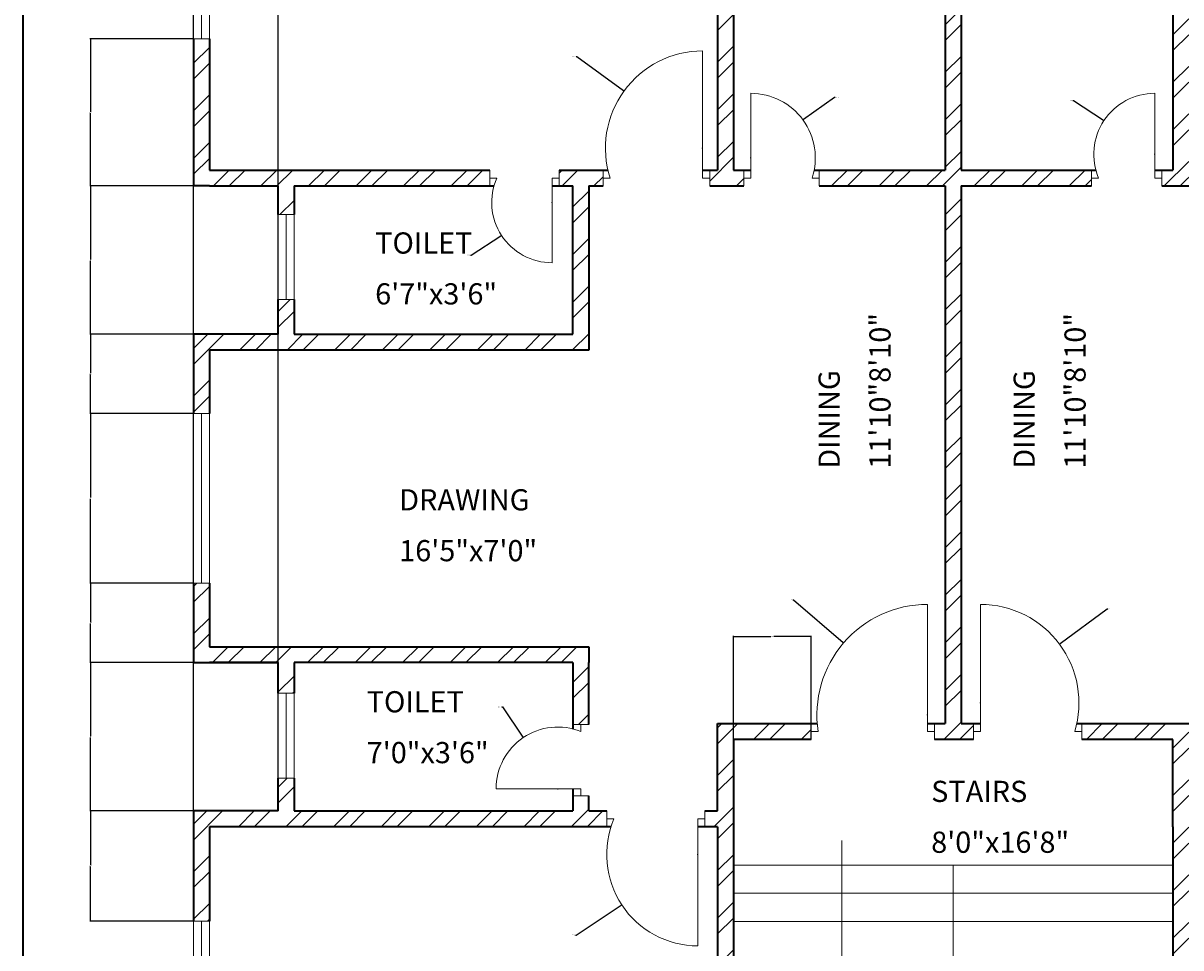
# Model space of a CAD drawing. Units: inches. Extents: x 2271 to 2815, y 1169 to 1838.
# Tile 2 of 4: x 2271 to 2599, y 1395 to 1657. Entities that reach past the tile are written whole.
import ezdxf

# ---------------------------------------------------------------- set-up
doc = ezdxf.new("R2010")
doc.units = ezdxf.units.IN
for name, color, linetype, lineweight in [('A-ANNO-DIMS', 2, 'Continuous', 18), ('A-ANNO-SYMB', 101, 'Continuous', 13), ('A-ANNO-TTLB', 7, 'Continuous', 35), ('A-AREA-IDEN', 7, 'Continuous', 18), ('A-DOOR', 11, 'Continuous', 18), ('A-FLOR-STRS', 101, 'Continuous', 18), ('A-GLAZ', 181, 'Continuous', 18), ('A-WALL', 7, 'Continuous', 35)]:
    doc.layers.add(name, color=color, linetype=linetype, lineweight=lineweight)
doc.layers.add('A-WALL-PATT', color=9, linetype='Continuous', lineweight=13, true_color=0xafd9aa)
doc.styles.get("Standard").update_dxf_attribs({"font": 'arial.ttf'})
doc.dimstyles.get("Standard").update_dxf_attribs({"dimtxt": 0.18, "dimasz": 0.18, "dimexe": 0.18, "dimexo": 0.0625, "dimgap": 0.09, "dimtad": 0, "dimtih": 1, "dimtoh": 1, "dimdec": 4, "dimzin": 0, "dimdsep": 46, "dimtxsty": 'Standard', "dimcen": 0.09, "dimadec": 0, "dimazin": 0, "dimtfac": 1, "dimtdec": 4, "dimtofl": 0, "dimtmove": 0, "dimatfit": 3, "dimfxl": 1, "dimtolj": 1, "dimtzin": 0, "dimarcsym": 0})

# ---------------------------------------------------------------- blocks, each defined once
blk = doc.blocks.new('WIN-60IN')
for p, q in [((0, 4.5), (0, 0)), ((60, 4.5), (0, 4.5)), ((60, 2.25), (60, 4.5)), ((60, 4.5), (60, 0)), ((0, 0), (0, 2.25)), ((0, 2.25), (60, 2.25)), ((0, 0), (60, 0))]:
    blk.add_line(p, q)
blk = doc.blocks.new('WIN-24IN')
for p, q in [((0, 4.5), (0, 0)), ((0, 4.5), (24, 4.5)), ((24, 2.25), (24, 4.5)), ((24, 4.5), (24, 0)), ((0, 0), (0, 2.25)), ((0, 2.25), (24, 2.25)), ((24, 0), (0, 0))]:
    blk.add_line(p, q)
blk = doc.blocks.new('*D14')
at = {"layer": 'A-ANNO-DIMS', "color": 0, "lineweight": -2, "transparency": 16777216}
for p, q in [((2318.74, 1433.53), (2289.47, 1433.53)), ((2289.65, 1433.35), (2289.65, 1418.1)), ((2289.65, 1402.49), (2289.65, 1417.74)), ((2318.74, 1402.31), (2289.47, 1402.31))]:
    blk.add_line(p, q, dxfattribs=at)
at = {"layer": 'A-ANNO-DIMS', "color": 0, "transparency": 16777216}
for points in [[(2289.62, 1433.35), (2289.68, 1433.35), (2289.65, 1433.53)], [(2289.62, 1402.49), (2289.68, 1402.49), (2289.65, 1402.31)]]:
    blk.add_solid(points, dxfattribs=at)
at = {"layer": 'Defpoints', "color": 0, "transparency": 16777216}
for p in [(2289.65, 1433.53), (2318.8, 1433.53), (2318.8, 1402.31)]:
    blk.add_point(p, dxfattribs=at)
at = {"layer": 'A-ANNO-DIMS', "color": 0, "transparency": 16777216, "insert": (2289.65, 1417.92), "char_height": 0.18, "attachment_point": 5}
blk.add_mtext('\\A1;31.22', dxfattribs=at)
blk = doc.blocks.new('*D15')
at = {"layer": 'A-ANNO-DIMS', "color": 0, "lineweight": -2, "transparency": 16777216}
for p, q in [((2318.74, 1475.53), (2289.47, 1475.53)), ((2289.65, 1475.35), (2289.65, 1454.71)), ((2289.65, 1433.71), (2289.65, 1454.35)), ((2318.74, 1433.53), (2289.47, 1433.53))]:
    blk.add_line(p, q, dxfattribs=at)
at = {"layer": 'A-ANNO-DIMS', "color": 0, "transparency": 16777216}
for points in [[(2289.62, 1475.35), (2289.68, 1475.35), (2289.65, 1475.53)], [(2289.62, 1433.71), (2289.68, 1433.71), (2289.65, 1433.53)]]:
    blk.add_solid(points, dxfattribs=at)
at = {"layer": 'Defpoints', "color": 0, "transparency": 16777216}
for p in [(2289.65, 1475.53), (2318.8, 1475.53), (2318.8, 1433.53)]:
    blk.add_point(p, dxfattribs=at)
at = {"layer": 'A-ANNO-DIMS', "color": 0, "transparency": 16777216, "insert": (2289.65, 1454.53), "char_height": 0.18, "attachment_point": 5}
blk.add_mtext('\\A1;42', dxfattribs=at)
blk = doc.blocks.new('*D16')
at = {"layer": 'A-ANNO-DIMS', "color": 0, "lineweight": -2, "transparency": 16777216}
for p, q in [((2318.74, 1498.07), (2289.47, 1498.07)), ((2289.65, 1497.89), (2289.65, 1486.98)), ((2289.65, 1475.71), (2289.65, 1486.62)), ((2318.74, 1475.53), (2289.47, 1475.53))]:
    blk.add_line(p, q, dxfattribs=at)
at = {"layer": 'A-ANNO-DIMS', "color": 0, "transparency": 16777216}
for points in [[(2289.62, 1497.89), (2289.68, 1497.89), (2289.65, 1498.07)], [(2289.62, 1475.71), (2289.68, 1475.71), (2289.65, 1475.53)]]:
    blk.add_solid(points, dxfattribs=at)
at = {"layer": 'Defpoints', "color": 0, "transparency": 16777216}
for p in [(2289.65, 1498.07), (2318.8, 1498.07), (2318.8, 1475.53)]:
    blk.add_point(p, dxfattribs=at)
at = {"layer": 'A-ANNO-DIMS', "color": 0, "transparency": 16777216, "insert": (2289.65, 1486.8), "char_height": 0.18, "attachment_point": 5}
blk.add_mtext('\\A1;22.54', dxfattribs=at)
blk = doc.blocks.new('*D17')
at = {"layer": 'A-ANNO-DIMS', "color": 0, "lineweight": -2, "transparency": 16777216}
for p, q in [((2318.74, 1546.07), (2289.47, 1546.07)), ((2289.65, 1545.89), (2289.65, 1522.25)), ((2289.65, 1498.25), (2289.65, 1521.89)), ((2318.74, 1498.07), (2289.47, 1498.07))]:
    blk.add_line(p, q, dxfattribs=at)
at = {"layer": 'A-ANNO-DIMS', "color": 0, "transparency": 16777216}
for points in [[(2289.62, 1545.89), (2289.68, 1545.89), (2289.65, 1546.07)], [(2289.62, 1498.25), (2289.68, 1498.25), (2289.65, 1498.07)]]:
    blk.add_solid(points, dxfattribs=at)
at = {"layer": 'Defpoints', "color": 0, "transparency": 16777216}
for p in [(2289.65, 1546.07), (2318.8, 1546.07), (2318.8, 1498.07)]:
    blk.add_point(p, dxfattribs=at)
at = {"layer": 'A-ANNO-DIMS', "color": 0, "transparency": 16777216, "insert": (2289.65, 1522.07), "char_height": 0.18, "attachment_point": 5}
blk.add_mtext('\\A1;48', dxfattribs=at)
blk = doc.blocks.new('*D18')
at = {"layer": 'A-ANNO-DIMS', "color": 0, "lineweight": -2, "transparency": 16777216}
for p, q in [((2318.74, 1568.53), (2289.47, 1568.53)), ((2289.65, 1568.35), (2289.65, 1557.48)), ((2289.65, 1546.25), (2289.65, 1557.12)), ((2318.74, 1546.07), (2289.47, 1546.07))]:
    blk.add_line(p, q, dxfattribs=at)
at = {"layer": 'A-ANNO-DIMS', "color": 0, "transparency": 16777216}
for points in [[(2289.62, 1568.35), (2289.68, 1568.35), (2289.65, 1568.53)], [(2289.62, 1546.25), (2289.68, 1546.25), (2289.65, 1546.07)]]:
    blk.add_solid(points, dxfattribs=at)
at = {"layer": 'Defpoints', "color": 0, "transparency": 16777216}
for p in [(2289.65, 1568.53), (2318.8, 1568.53), (2318.8, 1546.07)]:
    blk.add_point(p, dxfattribs=at)
at = {"layer": 'A-ANNO-DIMS', "color": 0, "transparency": 16777216, "insert": (2289.65, 1557.3), "char_height": 0.18, "attachment_point": 5}
blk.add_mtext('\\A1;22.46', dxfattribs=at)
blk = doc.blocks.new('*D19')
at = {"layer": 'A-ANNO-DIMS', "color": 0, "lineweight": -2, "transparency": 16777216}
for p, q in [((2318.74, 1610.53), (2289.47, 1610.53)), ((2289.65, 1610.35), (2289.65, 1589.71)), ((2289.65, 1568.71), (2289.65, 1589.35)), ((2318.74, 1568.53), (2289.47, 1568.53))]:
    blk.add_line(p, q, dxfattribs=at)
at = {"layer": 'A-ANNO-DIMS', "color": 0, "transparency": 16777216}
for points in [[(2289.62, 1610.35), (2289.68, 1610.35), (2289.65, 1610.53)], [(2289.62, 1568.71), (2289.68, 1568.71), (2289.65, 1568.53)]]:
    blk.add_solid(points, dxfattribs=at)
at = {"layer": 'Defpoints', "color": 0, "transparency": 16777216}
for p in [(2289.65, 1610.53), (2318.8, 1610.53), (2318.8, 1568.53)]:
    blk.add_point(p, dxfattribs=at)
at = {"layer": 'A-ANNO-DIMS', "color": 0, "transparency": 16777216, "insert": (2289.65, 1589.53), "char_height": 0.18, "attachment_point": 5}
blk.add_mtext('\\A1;42', dxfattribs=at)
blk = doc.blocks.new('*D20')
at = {"layer": 'A-ANNO-DIMS', "color": 0, "lineweight": -2, "transparency": 16777216}
for p, q in [((2318.74, 1652.22), (2289.47, 1652.22)), ((2289.65, 1652.04), (2289.65, 1631.56)), ((2289.65, 1610.71), (2289.65, 1631.19)), ((2318.74, 1610.53), (2289.47, 1610.53))]:
    blk.add_line(p, q, dxfattribs=at)
at = {"layer": 'A-ANNO-DIMS', "color": 0, "transparency": 16777216}
for points in [[(2289.62, 1652.04), (2289.68, 1652.04), (2289.65, 1652.22)], [(2289.62, 1610.71), (2289.68, 1610.71), (2289.65, 1610.53)]]:
    blk.add_solid(points, dxfattribs=at)
at = {"layer": 'Defpoints', "color": 0, "transparency": 16777216}
for p in [(2289.65, 1652.22), (2318.8, 1652.22), (2318.8, 1610.53)]:
    blk.add_point(p, dxfattribs=at)
at = {"layer": 'A-ANNO-DIMS', "color": 0, "transparency": 16777216, "insert": (2289.65, 1631.37), "char_height": 0.18, "attachment_point": 5}
blk.add_mtext('\\A1;41.69', dxfattribs=at)
blk = doc.blocks.new('*D23')
at = {"layer": 'A-ANNO-DIMS', "color": 0, "lineweight": -2, "transparency": 16777216}
for p, q in [((2318.8, 1433.59), (2318.8, 1816.86)), ((2318.98, 1816.68), (2330.58, 1816.68)), ((2342.62, 1816.68), (2331.02, 1816.68)), ((2342.8, 1433.59), (2342.8, 1816.86))]:
    blk.add_line(p, q, dxfattribs=at)
at = {"layer": 'A-ANNO-DIMS', "color": 0, "transparency": 16777216}
for points in [[(2318.98, 1816.71), (2318.98, 1816.65), (2318.8, 1816.68)], [(2342.62, 1816.71), (2342.62, 1816.65), (2342.8, 1816.68)]]:
    blk.add_solid(points, dxfattribs=at)
at = {"layer": 'Defpoints', "color": 0, "transparency": 16777216}
for p in [(2342.8, 1816.68), (2318.8, 1433.53), (2342.8, 1433.53)]:
    blk.add_point(p, dxfattribs=at)
at = {"layer": 'A-ANNO-DIMS', "color": 0, "transparency": 16777216, "insert": (2330.8, 1816.68), "char_height": 0.18, "attachment_point": 5}
blk.add_mtext('\\A1;24', dxfattribs=at)
blk = doc.blocks.new('*D36')
at = {"layer": 'A-ANNO-DIMS', "color": 0, "lineweight": -2, "transparency": 16777216}
for p, q in [((2471.8, 1453.82), (2471.8, 1483.08)), ((2471.98, 1482.9), (2482.4, 1482.9)), ((2493.61, 1482.9), (2483.19, 1482.9)), ((2493.79, 1453.82), (2493.79, 1483.08))]:
    blk.add_line(p, q, dxfattribs=at)
at = {"layer": 'A-ANNO-DIMS', "color": 0, "transparency": 16777216}
for points in [[(2471.98, 1482.93), (2471.98, 1482.87), (2471.8, 1482.9)], [(2493.61, 1482.93), (2493.61, 1482.87), (2493.79, 1482.9)]]:
    blk.add_solid(points, dxfattribs=at)
at = {"layer": 'Defpoints', "color": 0, "transparency": 16777216}
for p in [(2493.79, 1482.9), (2471.8, 1453.75), (2493.79, 1453.75)]:
    blk.add_point(p, dxfattribs=at)
at = {"layer": 'A-ANNO-DIMS', "color": 0, "transparency": 16777216, "insert": (2482.8, 1482.9), "char_height": 0.18, "attachment_point": 5}
blk.add_mtext('\\A1;21.99', dxfattribs=at)
blk = doc.blocks.new('*D37')
at = {"layer": 'A-ANNO-DIMS', "color": 0, "lineweight": -2, "transparency": 16777216}
for p, q in [((2488.58, 1493.35), (2488.76, 1493.35)), ((2488.76, 1493.35), (2502.87, 1481.23)), ((2526.65, 1460.7), (2526.83, 1460.7)), ((2526.74, 1460.61), (2526.74, 1460.79))]:
    blk.add_line(p, q, dxfattribs=at)
at = {"layer": 'A-ANNO-DIMS', "color": 0, "transparency": 16777216}
blk.add_solid([(2502.89, 1481.25), (2502.85, 1481.2), (2503, 1481.11)], dxfattribs=at)
at = {"layer": 'Defpoints', "color": 0, "transparency": 16777216}
for p in [(2503, 1481.11), (2526.74, 1460.7)]:
    blk.add_point(p, dxfattribs=at)
at = {"layer": 'A-ANNO-DIMS', "color": 0, "transparency": 16777216, "insert": (2488.03, 1493.35), "char_height": 0.18, "attachment_point": 5}
blk.add_mtext('\\A1;R31.305', dxfattribs=at)
blk = doc.blocks.new('*D38')
at = {"layer": 'A-ANNO-DIMS', "color": 0, "lineweight": -2, "transparency": 16777216}
for p, q in [((2577.64, 1490.7), (2564.34, 1480.83)), ((2577.82, 1490.7), (2577.64, 1490.7)), ((2541.69, 1464.1), (2541.87, 1464.1)), ((2541.78, 1464.01), (2541.78, 1464.19))]:
    blk.add_line(p, q, dxfattribs=at)
at = {"layer": 'A-ANNO-DIMS', "color": 0, "transparency": 16777216}
blk.add_solid([(2564.32, 1480.86), (2564.35, 1480.81), (2564.19, 1480.73)], dxfattribs=at)
at = {"layer": 'Defpoints', "color": 0, "transparency": 16777216}
for p in [(2564.19, 1480.73), (2541.78, 1464.1)]:
    blk.add_point(p, dxfattribs=at)
at = {"layer": 'A-ANNO-DIMS', "color": 0, "transparency": 16777216, "insert": (2578.23, 1490.7), "char_height": 0.18, "attachment_point": 5}
blk.add_mtext('\\A1;R27.9', dxfattribs=at)
blk = doc.blocks.new('*D39')
at = {"layer": 'A-ANNO-DIMS', "color": 0, "lineweight": -2, "transparency": 16777216}
for p, q in [((2427.25, 1647.18), (2427.43, 1647.18)), ((2427.43, 1647.18), (2440.65, 1637.56)), ((2462.97, 1621.24), (2463.15, 1621.24)), ((2463.06, 1621.15), (2463.06, 1621.33))]:
    blk.add_line(p, q, dxfattribs=at)
at = {"layer": 'A-ANNO-DIMS', "color": 0, "transparency": 16777216}
blk.add_solid([(2440.67, 1637.58), (2440.63, 1637.53), (2440.79, 1637.45)], dxfattribs=at)
at = {"layer": 'Defpoints', "color": 0, "transparency": 16777216}
for p in [(2440.79, 1637.45), (2463.06, 1621.24)]:
    blk.add_point(p, dxfattribs=at)
at = {"layer": 'A-ANNO-DIMS', "color": 0, "transparency": 16777216, "insert": (2426.7, 1647.18), "char_height": 0.18, "attachment_point": 5}
blk.add_mtext('\\A1;R27.546', dxfattribs=at)
blk = doc.blocks.new('*D41')
at = {"layer": 'A-ANNO-DIMS', "color": 0, "lineweight": -2, "transparency": 16777216}
for p, q in [((2461.62, 1421.13), (2461.8, 1421.13)), ((2461.71, 1421.04), (2461.71, 1421.22)), ((2427.2, 1398.34), (2439.99, 1406.79)), ((2427.02, 1398.34), (2427.2, 1398.34))]:
    blk.add_line(p, q, dxfattribs=at)
at = {"layer": 'A-ANNO-DIMS', "color": 0, "transparency": 16777216}
blk.add_solid([(2439.98, 1406.81), (2440.01, 1406.76), (2440.14, 1406.89)], dxfattribs=at)
at = {"layer": 'Defpoints', "color": 0, "transparency": 16777216}
for p in [(2461.71, 1421.13), (2440.14, 1406.89)]:
    blk.add_point(p, dxfattribs=at)
at = {"layer": 'A-ANNO-DIMS', "color": 0, "transparency": 16777216, "insert": (2426.47, 1398.34), "char_height": 0.18, "attachment_point": 5}
blk.add_mtext('\\A1;R25.845', dxfattribs=at)
blk = doc.blocks.new('*D47')
at = {"layer": 'A-ANNO-DIMS', "color": 0, "lineweight": -2, "transparency": 16777216}
for p, q in [((2500.41, 1635.64), (2491.67, 1629.32)), ((2500.59, 1635.64), (2500.41, 1635.64)), ((2476.63, 1618.51), (2476.81, 1618.51)), ((2476.72, 1618.42), (2476.72, 1618.6))]:
    blk.add_line(p, q, dxfattribs=at)
at = {"layer": 'A-ANNO-DIMS', "color": 0, "transparency": 16777216}
blk.add_solid([(2491.66, 1629.34), (2491.69, 1629.3), (2491.53, 1629.22)], dxfattribs=at)
at = {"layer": 'Defpoints', "color": 0, "transparency": 16777216}
for p in [(2491.53, 1629.22), (2476.72, 1618.51)]:
    blk.add_point(p, dxfattribs=at)
at = {"layer": 'A-ANNO-DIMS', "color": 0, "transparency": 16777216, "insert": (2501.14, 1635.64), "char_height": 0.18, "attachment_point": 5}
blk.add_mtext('\\A1;R18.274', dxfattribs=at)
blk = doc.blocks.new('*D49')
at = {"layer": 'A-ANNO-DIMS', "color": 0, "lineweight": -2, "transparency": 16777216}
for p, q in [((2406.19, 1462.97), (2406.37, 1462.97)), ((2406.37, 1462.97), (2412.14, 1454.42)), ((2421.95, 1439.79), (2422.13, 1439.79)), ((2422.04, 1439.7), (2422.04, 1439.88))]:
    blk.add_line(p, q, dxfattribs=at)
at = {"layer": 'A-ANNO-DIMS', "color": 0, "transparency": 16777216}
blk.add_solid([(2412.17, 1454.44), (2412.12, 1454.41), (2412.24, 1454.27)], dxfattribs=at)
at = {"layer": 'Defpoints', "color": 0, "transparency": 16777216}
for p in [(2412.24, 1454.27), (2422.04, 1439.79)]:
    blk.add_point(p, dxfattribs=at)
at = {"layer": 'A-ANNO-DIMS', "color": 0, "transparency": 16777216, "insert": (2405.64, 1462.97), "char_height": 0.18, "attachment_point": 5}
blk.add_mtext('\\A1;R17.485', dxfattribs=at)
blk = doc.blocks.new('*D51')
at = {"layer": 'A-ANNO-DIMS', "color": 0, "lineweight": -2, "transparency": 16777216}
for p, q in [((2567.95, 1634.76), (2568.13, 1634.76)), ((2568.13, 1634.76), (2576.61, 1629.15)), ((2591.06, 1619.53), (2591.24, 1619.53)), ((2591.15, 1619.44), (2591.15, 1619.62))]:
    blk.add_line(p, q, dxfattribs=at)
at = {"layer": 'A-ANNO-DIMS', "color": 0, "transparency": 16777216}
blk.add_solid([(2576.63, 1629.18), (2576.6, 1629.13), (2576.76, 1629.05)], dxfattribs=at)
at = {"layer": 'Defpoints', "color": 0, "transparency": 16777216}
for p in [(2576.76, 1629.05), (2591.15, 1619.53)]:
    blk.add_point(p, dxfattribs=at)
at = {"layer": 'A-ANNO-DIMS', "color": 0, "transparency": 16777216, "insert": (2567.47, 1634.76), "char_height": 0.18, "attachment_point": 5}
blk.add_mtext('\\A1;R17.25', dxfattribs=at)
blk = doc.blocks.new('*D52')
at = {"layer": 'A-ANNO-DIMS', "color": 0, "lineweight": -2, "transparency": 16777216}
for p, q in [((2420.3, 1605.88), (2420.48, 1605.88)), ((2420.39, 1605.79), (2420.39, 1605.97)), ((2397.48, 1590.94), (2405.92, 1596.45)), ((2397.3, 1590.94), (2397.48, 1590.94))]:
    blk.add_line(p, q, dxfattribs=at)
at = {"layer": 'A-ANNO-DIMS', "color": 0, "transparency": 16777216}
blk.add_solid([(2405.9, 1596.47), (2405.94, 1596.42), (2406.07, 1596.54)], dxfattribs=at)
at = {"layer": 'Defpoints', "color": 0, "transparency": 16777216}
for p in [(2420.39, 1605.88), (2406.07, 1596.54)]:
    blk.add_point(p, dxfattribs=at)
at = {"layer": 'A-ANNO-DIMS', "color": 0, "transparency": 16777216, "insert": (2396.75, 1590.94), "char_height": 0.18, "attachment_point": 5}
blk.add_mtext('\\A1;R17.095', dxfattribs=at)

msp = doc.modelspace()

# ---------------------------------------------------------------- hatches: boundary and pattern name
at = {"layer": 'A-WALL-PATT'}
h = msp.add_hatch(dxfattribs=at)
h.set_pattern_fill('ANSI32', color=256)
h.paths.add_polyline_path([(2441.4917, 1751.5314), (2397.0578, 1751.5314), (2397.0578, 1747.0314), (2441.4917, 1747.0314), (2441.4917, 1749.2814)])
h.paths.add_polyline_path([(2471.8006, 1787.5314), (2467.3006, 1787.5314), (2467.3006, 1783.0314), (2467.3006, 1751.5314), (2463.4131, 1751.5314), (2463.4131, 1747.0314), (2467.3006, 1747.0314), (2467.3006, 1615.0314), (2465.0606, 1615.0314), (2465.0606, 1610.5314), (2474.7192, 1610.5314), (2474.7192, 1612.7814), (2474.7192, 1615.0314), (2471.8006, 1615.0314), (2471.8006, 1747.0314), (2482.8275, 1747.0314), (2482.8275, 1749.2814), (2482.8275, 1751.5314), (2471.8006, 1751.5314)])
h.paths.add_polyline_path([(2549.5185, 1751.5314), (2506.8275, 1751.5314), (2506.8275, 1747.0314), (2531.8006, 1747.0314), (2531.8006, 1615.0314), (2496.0724, 1615.0314), (2496.0724, 1610.5314), (2531.8006, 1610.5314), (2531.8006, 1458.2548), (2528.7405, 1458.2548), (2528.7405, 1453.7548), (2539.7806, 1453.7548), (2539.7806, 1456.0048), (2539.7806, 1458.2548), (2536.3006, 1458.2548), (2536.3006, 1610.5314), (2573.267, 1610.5314), (2573.267, 1612.5736), (2573.267, 1612.7912), (2573.267, 1615.0314), (2536.3006, 1615.0314), (2536.3006, 1747.0314), (2549.5185, 1747.0314)])
h.paths.add_polyline_path([(2600.8006, 1787.5314), (2596.3006, 1787.5314), (2596.3006, 1747.0314), (2596.3006, 1615.0314), (2593.1473, 1615.0314), (2593.1473, 1610.5314), (2603.416, 1610.5314), (2603.416, 1612.7814), (2603.416, 1615.0314), (2600.8006, 1615.0314), (2600.8006, 1747.0314), (2603.7892, 1747.0314), (2603.7892, 1749.2814), (2603.7892, 1751.5314), (2600.8006, 1751.5314)])
h.paths.add_polyline_path([(2596.3006, 1751.5314), (2573.5185, 1751.5314), (2573.5185, 1747.0314), (2596.3006, 1747.0314)])
h.paths.add_polyline_path([(2648.9302, 1749.2814), (2648.9302, 1751.5314), (2624.6394, 1751.5314), (2624.6394, 1747.0314), (2648.9302, 1747.0314)])
h.paths.add_polyline_path([(2749.3006, 1751.5314), (2749.3006, 1787.5314), (2744.8006, 1787.5314), (2744.8006, 1751.5314), (2708.9302, 1751.5314), (2708.9302, 1747.0314), (2744.8006, 1747.0314), (2744.8006, 1715.8571), (2749.3006, 1715.8571)])
h.paths.add_polyline_path([(2337.0578, 1749.2814), (2337.0578, 1751.5314), (2323.3006, 1751.5314), (2323.3006, 1787.5314), (2318.8006, 1787.5314), (2318.8006, 1751.5314), (2318.8006, 1712.2179), (2323.3006, 1712.2179), (2323.3006, 1747.0314), (2337.0578, 1747.0314)])
h.paths.add_polyline_path([(2402.757, 1615.0314), (2323.3006, 1615.0314), (2323.3006, 1652.2179), (2318.8006, 1652.2179), (2318.8006, 1610.5314), (2323.3006, 1610.5314), (2342.8006, 1610.5314), (2342.8006, 1602.42), (2347.3006, 1602.42), (2347.3006, 1610.5314), (2402.757, 1610.5314)])
h.paths.add_polyline_path([(2430.8006, 1568.5314), (2430.8006, 1610.5314), (2434.8435, 1610.5314), (2434.8435, 1612.7814), (2434.8435, 1615.0314), (2422.3947, 1615.0314), (2422.3947, 1612.7814), (2422.3947, 1610.5314), (2426.3006, 1610.5314), (2426.3006, 1568.5314), (2347.3006, 1568.5314), (2347.3006, 1578.42), (2342.8006, 1578.42), (2342.8006, 1568.5314), (2318.8006, 1568.5314), (2318.8006, 1546.0693), (2322.7121, 1546.0693), (2323.3006, 1546.0693), (2323.3006, 1564.0314), (2342.8006, 1564.0314), (2347.3006, 1564.0314), (2430.8006, 1564.0314)])
h.paths.add_polyline_path([(2430.8006, 1480.0314), (2323.3006, 1480.0314), (2323.3006, 1498.0693), (2321.0506, 1498.0693), (2318.8006, 1498.0693), (2318.8006, 1475.5314), (2342.8006, 1475.5314), (2342.8006, 1466.8218), (2347.3006, 1466.8218), (2347.3006, 1475.5314), (2426.3006, 1475.5314), (2426.3006, 1458.0149), (2430.8006, 1458.0149), (2430.8006, 1475.5314)])
h.paths.add_polyline_path([(2435.9471, 1433.5314), (2430.8006, 1433.5314), (2430.8006, 1437.7896), (2426.3006, 1437.7896), (2426.3006, 1433.5314), (2347.3006, 1433.5314), (2347.3006, 1442.8218), (2342.8006, 1442.8218), (2342.8006, 1433.5314), (2318.8006, 1433.5314), (2318.8006, 1402.3145), (2323.3006, 1402.3145), (2323.3006, 1429.0314), (2342.8006, 1429.0314), (2347.3006, 1429.0314), (2435.9471, 1429.0314)])
h.paths.add_polyline_path([(2323.3006, 1342.3145), (2321.0506, 1342.3145), (2318.8006, 1342.3145), (2318.8006, 1304.5314), (2318.8006, 1268.5314), (2323.3006, 1268.5314), (2323.3006, 1304.5314), (2333.4662, 1304.5314), (2333.4662, 1306.7814), (2333.4662, 1309.0314), (2323.3006, 1309.0314)])
h.paths.add_polyline_path([(2437.8933, 1306.7814), (2437.8933, 1309.0314), (2393.4662, 1309.0314), (2393.4662, 1304.5314), (2437.8933, 1304.5314)])
h.paths.add_polyline_path([(2471.8006, 1453.7548), (2493.7895, 1453.7548), (2493.7895, 1456.0048), (2493.7895, 1458.2548), (2467.3006, 1458.2548), (2467.3006, 1433.5314), (2463.7134, 1433.5314), (2463.7134, 1431.2814), (2463.7134, 1429.0314), (2467.3006, 1429.0314), (2467.3006, 1309.0314), (2462.3197, 1309.0314), (2462.3197, 1304.5314), (2467.3006, 1304.5314), (2467.3006, 1268.5314), (2471.8006, 1268.5314), (2495.9201, 1268.5314), (2495.9201, 1270.7814), (2495.9201, 1273.0314), (2471.8006, 1273.0314), (2471.8006, 1309.0314)])
h.paths.add_polyline_path([(2600.8006, 1458.2548), (2570.4818, 1458.2548), (2570.4818, 1453.7548), (2596.3006, 1453.7548), (2596.3006, 1429.0314), (2596.3006, 1273.0314), (2555.9201, 1273.0314), (2555.9201, 1268.5314), (2596.3006, 1268.5314), (2600.8006, 1268.5314), (2600.8006, 1304.5314), (2604.5593, 1304.5314), (2604.5593, 1306.7814), (2604.5593, 1309.0314), (2600.8006, 1309.0314), (2600.8006, 1429.0314)])
h.paths.add_polyline_path([(2667.0861, 1309.0314), (2627.2, 1309.0314), (2627.2, 1304.5314), (2667.0861, 1304.5314)])
h.paths.add_polyline_path([(2749.3006, 1309.0314), (2749.3006, 1337.3095), (2744.8006, 1337.3095), (2744.8006, 1309.0314), (2727.0861, 1309.0314), (2727.0861, 1306.7814), (2727.0861, 1304.5314), (2744.8006, 1304.5314), (2744.8006, 1268.5314), (2749.3006, 1268.5314), (2749.3006, 1304.5314)])
h.paths.add_polyline_path([(2749.3006, 1433.5314), (2725.3006, 1433.5314), (2725.3006, 1442.7202), (2720.8006, 1442.7202), (2720.8006, 1433.5314), (2636.8006, 1433.5314), (2636.8006, 1437.8287), (2634.5506, 1437.8287), (2632.3006, 1437.8287), (2632.3006, 1433.5314), (2630.1129, 1433.5314), (2630.1129, 1429.0314), (2744.8006, 1429.0314), (2744.8006, 1397.3095), (2749.3006, 1397.3095)])
h.paths.add_polyline_path([(2749.3006, 1480.0314), (2749.3006, 1502.0415), (2744.8006, 1502.0415), (2744.8006, 1480.0314), (2720.8006, 1480.0314), (2632.3006, 1480.0314), (2632.3006, 1457.7851), (2636.8006, 1457.7851), (2636.8006, 1475.5314), (2720.8006, 1475.5314), (2720.8006, 1466.7202), (2725.3006, 1466.7202), (2725.3006, 1475.5314), (2749.3006, 1475.5314)])
h.paths.add_polyline_path([(2749.3006, 1568.5314), (2725.3006, 1568.5314), (2725.3006, 1578.9125), (2720.8006, 1578.9125), (2720.8006, 1568.5314), (2641.8006, 1568.5314), (2641.8006, 1610.5314), (2645.4823, 1610.5314), (2645.4823, 1612.7814), (2645.4823, 1615.0314), (2631.895, 1615.0314), (2631.895, 1610.5314), (2637.3006, 1610.5314), (2637.3006, 1568.5314), (2637.3006, 1564.0314), (2720.8006, 1564.0314), (2725.3006, 1564.0314), (2744.8006, 1564.0314), (2744.8006, 1550.0415), (2747.0506, 1550.0415), (2749.3006, 1550.0415)])
h.paths.add_polyline_path([(2749.3006, 1655.8571), (2744.8006, 1655.8571), (2744.8006, 1615.0314), (2668.3453, 1615.0314), (2668.3453, 1610.5314), (2720.8006, 1610.5314), (2720.8006, 1602.9125), (2725.3006, 1602.9125), (2725.3006, 1610.5314), (2749.3006, 1610.5314)])
h.paths.add_polyline_path([(2512.9815, 1676.2212), (2512.9815, 1716.3099), (2486.1477, 1716.3099), (2486.1477, 1676.2212)], flags=9)

# ---------------------------------------------------------------- linework, layer by layer
at = {"layer": 'A-ANNO-SYMB'}
msp.add_line((2502.512, 1425.1721), (2502.512, 1299.2714), dxfattribs=at)
at = {"layer": 'A-ANNO-TTLB'}
msp.add_lwpolyline([(2270.5512, 1838.2339), (2814.8691, 1838.2339), (2814.8691, 1168.8883), (2270.5512, 1168.8883)], close=True, dxfattribs=at)
at = {"layer": 'A-DOOR'}
for p, q in [((2463.0606, 1612.7814), (2463.0606, 1648.7814)), ((2476.7192, 1612.7814), (2476.7192, 1636.7814)), ((2591.1473, 1612.7814), (2591.1473, 1636.7814)), ((2402.757, 1610.5314), (2402.757, 1615.0314)), ((2402.757, 1615.0314), (2402.757, 1612.7814)), ((2422.3947, 1610.5314), (2422.3947, 1615.0314)), ((2422.3947, 1615.0314), (2422.3947, 1612.7814)), ((2434.8435, 1615.0314), (2434.8435, 1610.5314)), ((2465.0606, 1615.0314), (2465.0606, 1610.5314)), ((2474.7192, 1615.0314), (2474.7192, 1610.5314)), ((2496.0724, 1615.0314), (2496.0724, 1610.5314)), ((2573.267, 1615.0314), (2573.267, 1611.2989)), ((2593.1473, 1615.0314), (2593.1473, 1610.5314)), ((2402.757, 1612.7814), (2404.757, 1612.7814)), ((2422.3947, 1612.7814), (2420.3947, 1612.7814)), ((2420.3947, 1612.7814), (2420.3947, 1588.7814)), ((2434.8435, 1610.5314), (2434.8435, 1612.7814)), ((2434.8435, 1612.7814), (2436.8435, 1612.7814)), ((2465.0606, 1612.7814), (2463.0606, 1612.7814)), ((2465.0606, 1610.5314), (2465.0606, 1612.7814)), ((2474.7192, 1610.5314), (2474.7192, 1612.7814)), ((2474.7192, 1612.7814), (2476.7192, 1612.7814)), ((2496.0724, 1612.7814), (2494.0724, 1612.7814)), ((2496.0724, 1610.5314), (2496.0724, 1612.7814)), ((2573.267, 1612.5736), (2573.267, 1612.7912)), ((2573.267, 1612.7912), (2575.267, 1612.7912)), ((2573.267, 1610.5314), (2573.267, 1612.5736)), ((2573.267, 1611.2989), (2573.267, 1610.5314)), ((2593.1473, 1612.7814), (2591.1473, 1612.7814)), ((2593.1473, 1610.5314), (2593.1473, 1612.7814)), ((2526.7405, 1456.0048), (2526.7405, 1492.0048)), ((2541.7806, 1456.0048), (2541.7806, 1492.0048)), ((2426.3006, 1458.0149), (2430.8006, 1458.0149)), ((2430.8006, 1458.0149), (2428.5506, 1458.0149)), ((2428.5506, 1458.0149), (2428.5506, 1456.0149)), ((2493.7895, 1458.2548), (2493.7895, 1453.7548)), ((2528.7405, 1458.2548), (2528.7405, 1453.7548)), ((2539.7806, 1458.2548), (2539.7806, 1453.7548)), ((2570.4818, 1458.2548), (2570.4818, 1453.7548)), ((2493.7895, 1453.7548), (2493.7895, 1456.0048)), ((2493.7895, 1456.0048), (2495.7895, 1456.0048)), ((2528.7405, 1456.0048), (2526.7405, 1456.0048)), ((2528.7405, 1453.7548), (2528.7405, 1456.0048)), ((2539.7806, 1453.7548), (2539.7806, 1456.0048)), ((2539.7806, 1456.0048), (2541.7806, 1456.0048)), ((2570.4818, 1456.0048), (2568.4818, 1456.0048)), ((2570.4818, 1453.7548), (2570.4818, 1456.0048)), ((2428.5506, 1439.7896), (2404.5506, 1439.7896)), ((2426.3006, 1437.7896), (2430.8006, 1437.7896)), ((2430.8006, 1437.7896), (2426.3006, 1437.7896)), ((2426.3006, 1437.7896), (2428.5506, 1437.7896)), ((2428.5506, 1437.7896), (2428.5506, 1439.7896)), ((2435.9471, 1429.0314), (2435.9471, 1433.5314)), ((2435.9471, 1433.5314), (2435.9471, 1431.2814)), ((2463.7134, 1429.0314), (2463.7134, 1433.5314)), ((2463.7134, 1433.5314), (2463.7134, 1431.2814)), ((2435.9471, 1431.2814), (2437.9471, 1431.2814)), ((2463.7134, 1431.2814), (2461.7134, 1431.2814)), ((2461.7134, 1431.2814), (2461.7134, 1395.2814))]:
    msp.add_line(p, q, dxfattribs=at)
for centre, radius, start, end in [((2463.0606, 1621.2351), 27.5463, 90, 197.871943), ((2476.7192, 1618.5078), 18.2736, 341.73758, 90), ((2591.1473, 1619.5304), 17.251, 90, 202.99512), ((2420.3947, 1605.8759), 17.0945, 156.17402, 270), ((2526.7405, 1460.6998), 31.3051, 90, 188.62536), ((2541.7806, 1464.1027), 27.9021, 343.128628, 90), ((2422.0352, 1439.7896), 17.4846, 68.121867, 180), ((2461.7134, 1421.1264), 25.845, 156.863691, 270)]:
    msp.add_arc(centre, radius, start, end, dxfattribs=at)
at = {"layer": 'A-FLOR-STRS'}
for p, q in [((2471.8006, 1418.1711), (2596.3006, 1418.1711)), ((2534.0506, 1314.1711), (2534.0506, 1418.1711)), ((2471.8006, 1410.1711), (2596.3006, 1410.1711)), ((2471.8006, 1402.1711), (2596.3006, 1402.1711))]:
    msp.add_line(p, q, dxfattribs=at)
at = {"layer": 'A-GLAZ'}
for p, q in [((2321.0506, 1546.0693), (2318.8006, 1546.0693)), ((2318.8006, 1546.0693), (2322.7121, 1546.0693)), ((2318.8006, 1546.0693), (2318.8006, 1498.0693)), ((2321.0506, 1498.0693), (2321.0506, 1546.0693)), ((2322.7121, 1546.0693), (2323.3006, 1546.0693)), ((2323.3006, 1498.0693), (2323.3006, 1546.0693)), ((2318.8006, 1498.0693), (2323.3006, 1498.0693)), ((2323.3006, 1498.0693), (2321.0506, 1498.0693)), ((2342.8006, 1466.8218), (2347.3006, 1466.8218)), ((2342.8006, 1442.8218), (2342.8006, 1466.8218)), ((2347.3006, 1466.8218), (2345.0506, 1466.8218)), ((2345.0506, 1466.8218), (2345.0506, 1442.8218)), ((2347.3006, 1466.8218), (2347.3006, 1442.8218)), ((2347.3006, 1442.8218), (2342.8006, 1442.8218)), ((2345.0506, 1442.8218), (2347.3006, 1442.8218))]:
    msp.add_line(p, q, dxfattribs=at)
at = {"layer": 'A-WALL'}
for p, q in [((2467.3006, 1747.0314), (2467.3006, 1615.0314)), ((2471.8006, 1747.0314), (2471.8006, 1615.0314)), ((2531.8006, 1747.0314), (2531.8006, 1615.0314)), ((2536.3006, 1747.0314), (2536.3006, 1615.0314)), ((2596.3006, 1747.0314), (2596.3006, 1615.0314)), ((2318.8006, 1652.2179), (2318.8006, 1610.5314)), ((2323.3006, 1652.2179), (2323.3006, 1615.0314)), ((2323.3006, 1615.0314), (2402.757, 1615.0314)), ((2422.3947, 1615.0314), (2436.2219, 1615.0314)), ((2463.0606, 1615.0314), (2467.3006, 1615.0314)), ((2471.8006, 1615.0314), (2476.7192, 1615.0314)), ((2494.6591, 1615.0314), (2531.8006, 1615.0314)), ((2536.3006, 1615.0314), (2574.4932, 1615.0314)), ((2591.1473, 1615.0314), (2596.3006, 1615.0314)), ((2323.3006, 1610.5314), (2318.8006, 1610.5314)), ((2323.3006, 1610.5314), (2342.8006, 1610.5314)), ((2323.3006, 1610.5314), (2342.8006, 1610.5314)), ((2342.8006, 1602.42), (2342.8006, 1610.5314)), ((2347.3006, 1610.5314), (2347.3006, 1602.42)), ((2347.3006, 1610.5314), (2403.9463, 1610.5314)), ((2420.3947, 1610.5314), (2426.3006, 1610.5314)), ((2426.3006, 1568.5314), (2426.3006, 1610.5314)), ((2430.8006, 1610.5314), (2430.8006, 1568.5314)), ((2430.8006, 1610.5314), (2434.8435, 1610.5314)), ((2465.0606, 1610.5314), (2474.7192, 1610.5314)), ((2496.0724, 1610.5314), (2531.8006, 1610.5314)), ((2531.8006, 1610.5314), (2531.8006, 1458.2548)), ((2536.3006, 1610.5314), (2536.3006, 1458.2548)), ((2536.3006, 1610.5314), (2573.267, 1610.5314)), ((2593.1473, 1610.5314), (2603.416, 1610.5314)), ((2342.8006, 1568.5314), (2342.8006, 1578.42)), ((2347.3006, 1578.42), (2347.3006, 1568.5314)), ((2342.8006, 1568.5314), (2318.8006, 1568.5314)), ((2318.8006, 1568.5314), (2318.8006, 1546.0693)), ((2347.3006, 1568.5314), (2426.3006, 1568.5314)), ((2430.8006, 1568.5314), (2430.8006, 1564.0314)), ((2323.3006, 1564.0314), (2323.3006, 1546.0693)), ((2342.8006, 1564.0314), (2323.3006, 1564.0314)), ((2323.3006, 1564.0314), (2323.3006, 1546.0693)), ((2347.3006, 1564.0314), (2342.8006, 1564.0314)), ((2430.8006, 1564.0314), (2347.3006, 1564.0314)), ((2318.8006, 1498.0693), (2318.8006, 1475.5314)), ((2323.3006, 1498.0693), (2323.3006, 1480.0314)), ((2323.3006, 1498.0693), (2323.3006, 1480.0314)), ((2323.3006, 1480.0314), (2430.8006, 1480.0314)), ((2430.8006, 1480.0314), (2430.8006, 1475.5314)), ((2318.8006, 1475.5314), (2342.8006, 1475.5314)), ((2342.8006, 1475.5314), (2323.3006, 1475.5314)), ((2342.8006, 1466.8218), (2342.8006, 1475.5314)), ((2426.3006, 1475.5314), (2347.3006, 1475.5314)), ((2347.3006, 1475.5314), (2347.3006, 1466.8218)), ((2426.3006, 1475.5314), (2426.3006, 1456.746)), ((2430.8006, 1458.0149), (2430.8006, 1475.5314)), ((2467.3006, 1433.5314), (2467.3006, 1458.2548)), ((2467.3006, 1458.2548), (2495.531, 1458.2548)), ((2526.7405, 1458.2548), (2531.8006, 1458.2548)), ((2536.3006, 1458.2548), (2541.7806, 1458.2548)), ((2569.063, 1458.2548), (2600.8006, 1458.2548)), ((2471.8006, 1453.7548), (2471.8006, 1309.0314)), ((2471.8006, 1453.7548), (2471.8006, 1433.5314)), ((2493.7895, 1453.7548), (2471.8006, 1453.7548)), ((2539.7806, 1453.7548), (2528.7405, 1453.7548)), ((2596.3006, 1453.7548), (2570.4818, 1453.7548)), ((2596.3006, 1429.0314), (2596.3006, 1453.7548)), ((2342.8006, 1433.5314), (2342.8006, 1442.8218)), ((2347.3006, 1442.8218), (2347.3006, 1433.5314)), ((2426.3006, 1439.7896), (2426.3006, 1433.5314)), ((2430.8006, 1433.5314), (2430.8006, 1437.7896)), ((2342.8006, 1433.5314), (2318.8006, 1433.5314)), ((2318.8006, 1433.5314), (2318.8006, 1402.3145)), ((2347.3006, 1433.5314), (2426.3006, 1433.5314)), ((2347.3006, 1433.5314), (2426.3006, 1433.5314)), ((2430.8006, 1433.5314), (2435.9471, 1433.5314)), ((2430.8006, 1433.5314), (2435.9471, 1433.5314)), ((2463.7134, 1433.5314), (2467.3006, 1433.5314)), ((2463.7134, 1433.5314), (2467.3006, 1433.5314)), ((2323.3006, 1429.0314), (2323.3006, 1402.3145)), ((2342.8006, 1429.0314), (2323.3006, 1429.0314)), ((2323.3006, 1429.0314), (2323.3006, 1402.3145)), ((2347.3006, 1429.0314), (2342.8006, 1429.0314)), ((2437.107, 1429.0314), (2347.3006, 1429.0314)), ((2467.3006, 1429.0314), (2461.7134, 1429.0314)), ((2467.3006, 1429.0314), (2467.3006, 1309.0314)), ((2596.3006, 1429.0314), (2596.3006, 1273.0314))]:
    msp.add_line(p, q, dxfattribs=at)

# ---------------------------------------------------------------- block references
at = {"layer": 'A-GLAZ', "extrusion": (0, 0, -1), "zscale": -1, "rotation": 90}
for name, p in [('WIN-60IN', (-2318.8001, 1652.2181)), ('WIN-24IN', (-2342.8001, 1578.4195))]:
    msp.add_blockref(name, p, dxfattribs=at)
at = {"layer": 'A-GLAZ', "rotation": 90}
msp.add_blockref('WIN-60IN', (2323.301, 1342.3147), dxfattribs=at)

# ---------------------------------------------------------------- texts
at = {"layer": 'A-AREA-IDEN', "char_height": 6, "attachment_point": 1, "line_spacing_factor": 1.44}
for s, width, insert in [('TOILET\\P6\'7"x3\'6"', 98.703212, (2370.2837, 1597.3773)), ('DRAWING\\P16\'5"x7\'0"', 121.219978, (2377.089, 1524.6345)), ('TOILET\\P7\'0"x3\'6"', 128.894102, (2367.877, 1467.4291)), ('STAIRS\\P8\'0"x16\'8"', 75.661427, (2527.813, 1442.0471))]:
    msp.add_mtext_dynamic_manual_height_columns(s, width=width, gutter_width=12.5, heights=[0], dxfattribs=dict(at, insert=insert))
at = {"layer": 'A-AREA-IDEN', "char_height": 6, "attachment_point": 1, "rotation": 90, "line_spacing_factor": 1.44}
for insert in [(2495.904, 1530.4473), (2551.1703, 1530.4473)]:
    msp.add_mtext_dynamic_manual_height_columns('DINING\\P11\'10"8\'10"', width=92.119391, gutter_width=12.5, heights=[0], dxfattribs=dict(at, insert=insert))

# ---------------------------------------------------------------- dimensions: what is measured, and where the dimension line sits
at = {"layer": 'A-ANNO-DIMS'}
for base, p1, p2, override, picture, middle in [((2342.8006, 1816.6814), (2318.8006, 1433.5314), (2342.8006, 1433.5314), {"dimdec": 0, "dimlfac": 1, "dimrnd": 0, "dimzin": 0, "dimdsep": 46, "dimlunit": 2}, '*D23', (2330.8006, 1816.6814)), ((2493.7895, 1482.9048), (2471.8006, 1453.7548), (2493.7895, 1453.7548), {"dimdec": 2, "dimlfac": 1, "dimrnd": 0, "dimzin": 0, "dimdsep": 46, "dimlunit": 2}, '*D36', (2482.795, 1482.9048))]:
    dim = msp.add_linear_dim(base=base, p1=p1, p2=p2, dimstyle='Standard', override=override, dxfattribs=at)
    dim.commit()
    dim.dimension.update_dxf_attribs({"geometry": picture, "text_midpoint": middle})
for base, p1, p2, override, picture, middle in [((2289.6506, 1652.2179), (2318.8006, 1610.5314), (2318.8006, 1652.2179), {"dimdec": 2, "dimlfac": 1, "dimrnd": 0, "dimzin": 0, "dimdsep": 46, "dimlunit": 2}, '*D20', (2289.6506, 1631.3747)), ((2289.6506, 1610.5314), (2318.8006, 1568.5314), (2318.8006, 1610.5314), {"dimdec": 0, "dimlfac": 1, "dimrnd": 0, "dimzin": 0, "dimdsep": 46, "dimlunit": 2}, '*D19', (2289.6506, 1589.5314)), ((2289.6506, 1568.5314), (2318.8006, 1546.0693), (2318.8006, 1568.5314), {"dimdec": 2, "dimlfac": 1, "dimrnd": 0, "dimzin": 0, "dimdsep": 46, "dimlunit": 2}, '*D18', (2289.6506, 1557.3004)), ((2289.6506, 1546.0693), (2318.8006, 1498.0693), (2318.8006, 1546.0693), {"dimdec": 0, "dimlfac": 1, "dimrnd": 0, "dimzin": 0, "dimdsep": 46, "dimlunit": 2}, '*D17', (2289.6506, 1522.0693)), ((2289.6506, 1498.0693), (2318.8006, 1475.5314), (2318.8006, 1498.0693), {"dimdec": 2, "dimlfac": 1, "dimrnd": 0, "dimzin": 0, "dimdsep": 46, "dimlunit": 2}, '*D16', (2289.6506, 1486.8004)), ((2289.6506, 1475.5314), (2318.8006, 1433.5314), (2318.8006, 1475.5314), {"dimdec": 0, "dimlfac": 1, "dimrnd": 0, "dimzin": 0, "dimdsep": 46, "dimlunit": 2}, '*D15', (2289.6506, 1454.5314)), ((2289.6506, 1433.5314), (2318.8006, 1402.3145), (2318.8006, 1433.5314), {"dimdec": 2, "dimlfac": 1, "dimrnd": 0, "dimzin": 0, "dimdsep": 46, "dimlunit": 2}, '*D14', (2289.6506, 1417.923))]:
    dim = msp.add_linear_dim(base=base, p1=p1, p2=p2, angle=90, dimstyle='Standard', override=override, dxfattribs=at)
    dim.commit()
    dim.dimension.update_dxf_attribs({"geometry": picture, "text_midpoint": middle})
for center, mpoint, override, picture, middle in [((2463.0606, 1621.2351), (2440.793, 1637.451), {"dimdec": 3, "dimlfac": 1, "dimrnd": 0, "dimzin": 0, "dimdsep": 46, "dimlunit": 2}, '*D39', (2426.7028, 1647.1805)), ((2476.7192, 1618.5078), (2491.5272, 1629.2152), {"dimdec": 3, "dimlfac": 1, "dimrnd": 0, "dimzin": 0, "dimdsep": 46, "dimlunit": 2}, '*D47', (2501.1414, 1635.6396)), ((2591.1473, 1619.5304), (2576.762, 1629.052), {"dimdec": 2, "dimlfac": 1, "dimrnd": 0, "dimzin": 0, "dimdsep": 46, "dimlunit": 2}, '*D51', (2567.4703, 1634.765)), ((2420.3947, 1605.8759), (2406.072, 1596.544), {"dimdec": 3, "dimlfac": 1, "dimrnd": 0, "dimzin": 0, "dimdsep": 46, "dimlunit": 2}, '*D52', (2396.748, 1590.9449)), ((2526.7405, 1460.6998), (2503.003, 1481.109), {"dimdec": 3, "dimlfac": 1, "dimrnd": 0, "dimzin": 0, "dimdsep": 46, "dimlunit": 2}, '*D37', (2488.03, 1493.3546)), ((2541.7806, 1464.1027), (2564.191, 1480.725), {"dimdec": 1, "dimlfac": 1, "dimrnd": 0, "dimzin": 0, "dimdsep": 46, "dimlunit": 2}, '*D38', (2578.2274, 1490.6984)), ((2422.0352, 1439.7896), (2412.243, 1454.2749), {"dimdec": 3, "dimlfac": 1, "dimrnd": 0, "dimzin": 0, "dimdsep": 46, "dimlunit": 2}, '*D49', (2405.6373, 1462.9662)), ((2461.7134, 1421.1264), (2440.1449, 1406.8869), {"dimdec": 3, "dimlfac": 1, "dimrnd": 0, "dimzin": 0, "dimdsep": 46, "dimlunit": 2}, '*D41', (2426.4734, 1398.3433))]:
    dim = msp.add_radius_dim(center=center, mpoint=mpoint, dimstyle='Standard', override=override, dxfattribs=at)
    dim.commit()
    dim.dimension.update_dxf_attribs({"geometry": picture, "text_midpoint": middle, "dimtype": 164})

doc.saveas('drawing.dxf')
